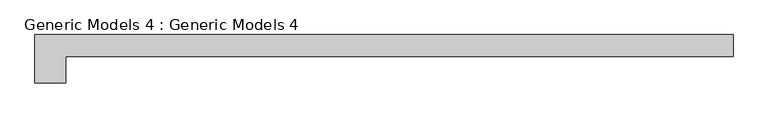
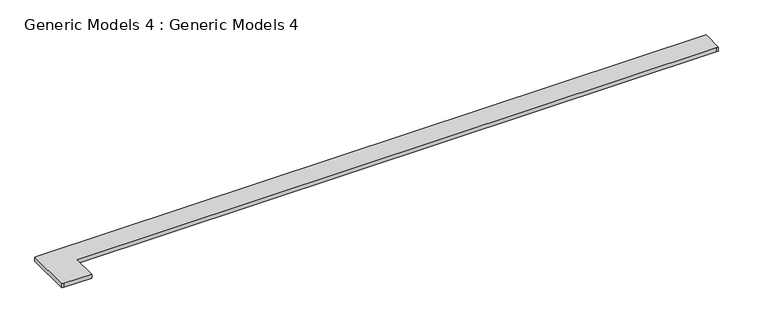
"""IFC4 building model written with IfcOpenShell, lengths in millimetres: proxy geometry, Generic Models 4 : Generic Models 4."""

from ifc_helpers import new_model, si_unit, frame, origin, place, context, project, spatial, polyline, outline, extrude, source, transform, mapped, element, save


def generic_models_4_generic_models_4_4063ad9d(model_context):
    return source(origin(), model_context, "Body", "SweptSolid", [
        extrude(outline(polyline([(-8151.9519453, 3641.8444012), (-8482.1519453, 3641.8444012), (-8507.5519453, 3641.8444012), (-8507.5519453, 4200.6444012), (-8482.1519453, 4200.6444012), (-474.8019453, 4200.6444012), (-474.8019453, 3946.6444012), (-500.2019453, 3946.6444012), (-8151.9519453, 3946.6444012), (-8151.9519453, 3641.8444012)])), frame((0.0, 0.0, 7010.4), z_axis=(0.0, 0.0, 1.0), x_axis=(1.0, 0.0, 0.0)), (0.0, 0.0, 1.0), 50.8),
    ])


if __name__ == "__main__":
    model = new_model("IFC4")
    model_context = context("Model", 3, world=origin())
    ifc_project = project(units=[si_unit("LENGTHUNIT", "METRE", prefix="MILLI")], contexts=[model_context])
    site = spatial("IfcSite", under=ifc_project)
    building = spatial("IfcBuilding", under=site)
    placement = place(None, origin())
    generic_models_4_generic_models_4_shape = generic_models_4_generic_models_4_4063ad9d(model_context)
    element("IfcBuildingElementProxy", 1, Name="Generic Models 4 : Generic Models 4", ObjectType="Generic Models 4 : Generic Models 4", at=placement, inside=building, context=model_context, shape_type="MappedRepresentation", body=[
        mapped(generic_models_4_generic_models_4_shape, transform((0.0, 0.0, 0.0), x_axis=(1.0, 0.0, 0.0), y_axis=(0.0, 1.0, 0.0), z_axis=(0.0, 0.0, 1.0))),
    ])
    save(model, "model.ifc")
